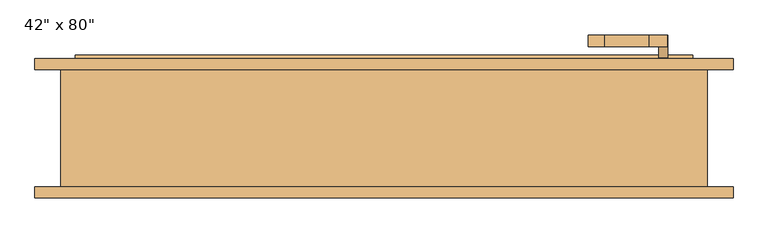
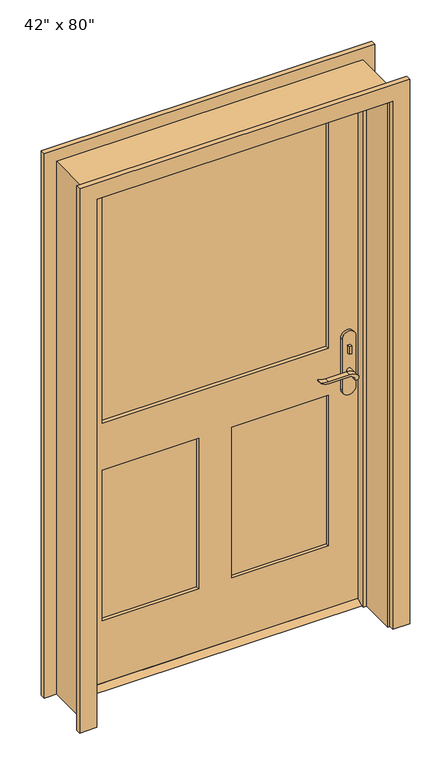
"""IFC4 building model written with IfcOpenShell, lengths in millimetres: door geometry."""

from ifc_helpers import new_model, si_unit, point, frame, frame_2d, origin, place, context, project, spatial, polyline, circle_curve, trimmed, segment, composite_curve, outline, extrude, faceted_brep, source, transform, mapped, element, save


def door_e0076512(model_context):
    return source(origin(), model_context, "Body", "SolidModel", [
        extrude(outline(polyline([(63.5, 12.7), (98.425, 12.7), (123.825, 0.0), (38.1, 0.0), (63.5, 12.7)])), frame((-533.4, 0.0, 0.0), z_axis=(1.0, 0.0, 0.0), x_axis=(0.0, 1.0, 0.0)), (0.0, 0.0, 1.0), 1066.8),
        extrude(outline(polyline([(487.6, 43.5), (477.6, 43.5), (477.6, 53.5), (487.6, 53.5), (487.6, 43.5)])), frame((0.0, 0.0, 981.9), z_axis=(0.0, 0.0, 1.0), x_axis=(1.0, 0.0, 0.0)), (0.0, 0.0, 1.0), 30.0),
        extrude(outline(composite_curve([segment(trimmed(circle_curve(frame_2d((996.9, 482.6)), 8.0), [point((996.9, 474.6))], [point((996.9, 490.6))], False, "CARTESIAN"), True, "CONTINUOUS"), segment(trimmed(circle_curve(frame_2d((996.9, 482.6)), 8.0), [point((996.9, 490.6))], [point((996.9, 474.6))], False, "CARTESIAN"), True, "CONTINUOUS")], self_intersect=False)), frame((0.0, 108.425, 0.0), z_axis=(0.0, 1.0, 0.0), x_axis=(0.0, 0.0, 1.0)), (0.0, 0.0, 1.0), 10.0),
        extrude(outline(composite_curve([segment(trimmed(circle_curve(frame_2d((897.1555521, 458.9324871)), 37.2832219), [point((919.0523287, 489.1081363))], [point((934.4, 457.2325667))], False, "CARTESIAN"), True, "CONTINUOUS"), segment(polyline([(934.4, 457.2325667), (934.4, 380.9564091)]), True, "CONTINUOUS"), segment(trimmed(circle_curve(frame_2d((1017.6850638, 381.0227909)), 83.2850902), [point((934.4, 380.9564091))], [point((939.4, 352.6))], True, "CARTESIAN"), True, "CONTINUOUS"), segment(polyline([(939.4, 352.6), (936.6135558, 352.6)]), True, "CONTINUOUS"), segment(trimmed(circle_curve(frame_2d((986.6709207, 384.5396612)), 59.3791355), [point((936.6135558, 352.6))], [point((927.4, 380.9564091))], False, "CARTESIAN"), True, "CONTINUOUS"), segment(polyline([(927.4, 380.9564091), (927.4, 457.2138099)]), True, "CONTINUOUS"), segment(trimmed(circle_curve(frame_2d((909.2738613, 457.2138099)), 18.1261387), [point((927.4, 457.2138099))], [point((914.4, 474.6))], True, "CARTESIAN"), True, "CONTINUOUS"), segment(trimmed(circle_curve(frame_2d((914.4, 482.6)), 8.0), [point((914.4, 474.6))], [point((919.0523287, 489.1081363))], False, "CARTESIAN"), True, "CONTINUOUS")], self_intersect=False)), frame((0.0, 3.5, 0.0), z_axis=(0.0, 1.0, 0.0), x_axis=(0.0, 0.0, 1.0)), (0.0, 0.0, 1.0), 20.0),
        extrude(outline(composite_curve([segment(trimmed(circle_curve(frame_2d((914.4, 482.6)), 8.0), [point((914.3999903, 474.6))], [point((919.0523287, 489.1081363))], False, "CARTESIAN"), True, "CONTINUOUS"), segment(trimmed(circle_curve(frame_2d((897.1555521, 458.9324871)), 37.2832219), [point((919.0523287, 489.1081363))], [point((934.4, 457.2325667))], False, "CARTESIAN"), True, "CONTINUOUS"), segment(polyline([(934.4, 457.2325667), (934.4, 380.9564091)]), True, "CONTINUOUS"), segment(trimmed(circle_curve(frame_2d((1017.6850638, 381.0227909)), 83.2850902), [point((934.4, 380.9564091))], [point((939.4, 352.6))], True, "CARTESIAN"), True, "CONTINUOUS"), segment(polyline([(939.4, 352.6), (936.6135558, 352.6)]), True, "CONTINUOUS"), segment(trimmed(circle_curve(frame_2d((986.6709207, 384.5396612)), 59.3791355), [point((936.6135558, 352.6))], [point((927.4, 380.9564091))], False, "CARTESIAN"), True, "CONTINUOUS"), segment(polyline([(927.4, 380.9564091), (927.4, 457.2138122)]), True, "CONTINUOUS"), segment(trimmed(circle_curve(frame_2d((909.2738682, 457.2138122)), 18.1261318), [point((927.4, 457.2138122))], [point((914.3999903, 474.6))], True, "CARTESIAN"), True, "CONTINUOUS")], self_intersect=False)), frame((0.0, 138.425, 0.0), z_axis=(0.0, 1.0, 0.0), x_axis=(0.0, 0.0, 1.0)), (0.0, 0.0, 1.0), 20.0),
        extrude(outline(composite_curve([segment(trimmed(circle_curve(frame_2d((914.4, 482.6)), 8.0), [point((914.4, 474.6))], [point((914.4, 490.6))], False, "CARTESIAN"), True, "CONTINUOUS"), segment(trimmed(circle_curve(frame_2d((914.4, 482.6)), 8.0), [point((914.4, 490.6))], [point((914.4, 474.6))], False, "CARTESIAN"), True, "CONTINUOUS")], self_intersect=False)), frame((0.0, 23.5, 0.0), z_axis=(0.0, 1.0, 0.0), x_axis=(0.0, 0.0, 1.0)), (0.0, 0.0, 1.0), 30.0),
        extrude(outline(composite_curve([segment(trimmed(circle_curve(frame_2d((914.4, 482.6)), 8.0), [point((914.4, 474.6))], [point((914.4, 490.6))], False, "CARTESIAN"), True, "CONTINUOUS"), segment(trimmed(circle_curve(frame_2d((914.4, 482.6)), 8.0), [point((914.4, 490.6))], [point((914.4, 474.6))], False, "CARTESIAN"), True, "CONTINUOUS")], self_intersect=False)), frame((0.0, 108.425, 0.0), z_axis=(0.0, 1.0, 0.0), x_axis=(0.0, 0.0, 1.0)), (0.0, 0.0, 1.0), 30.0),
        extrude(outline(composite_curve([segment(polyline([(844.4, 507.6), (1039.4, 507.6)]), True, "CONTINUOUS"), segment(trimmed(circle_curve(frame_2d((1039.4, 482.6)), 25.0), [point((1039.4, 507.6))], [point((1039.4, 457.6))], False, "CARTESIAN"), True, "CONTINUOUS"), segment(polyline([(1039.4, 457.6), (844.4, 457.6)]), True, "CONTINUOUS"), segment(trimmed(circle_curve(frame_2d((844.4, 482.6)), 25.0), [point((844.4, 457.6))], [point((844.4, 507.6))], False, "CARTESIAN"), True, "CONTINUOUS")], self_intersect=False)), frame((0.0, 53.5, 0.0), z_axis=(0.0, 1.0, 0.0), x_axis=(0.0, 0.0, 1.0)), (0.0, 0.0, 1.0), 10.0),
        extrude(outline(composite_curve([segment(polyline([(844.4, 507.6), (1039.4, 507.6)]), True, "CONTINUOUS"), segment(trimmed(circle_curve(frame_2d((1039.4, 482.6)), 25.0), [point((1039.4, 507.6))], [point((1039.4, 457.6))], False, "CARTESIAN"), True, "CONTINUOUS"), segment(polyline([(1039.4, 457.6), (844.4, 457.6)]), True, "CONTINUOUS"), segment(trimmed(circle_curve(frame_2d((844.4, 482.6)), 25.0), [point((844.4, 457.6))], [point((844.4, 507.6))], False, "CARTESIAN"), True, "CONTINUOUS")], self_intersect=False)), frame((0.0, 98.425, 0.0), z_axis=(0.0, 1.0, 0.0), x_axis=(0.0, 0.0, 1.0)), (0.0, 0.0, 1.0), 10.0),
        extrude(outline(polyline([(2032.0, -533.4), (12.7, -533.4), (12.7, 533.4), (2032.0, 533.4), (2032.0, -533.4)]), holes=[polyline([(1016.0, -412.75), (1911.35, -412.75), (1911.35, 412.75), (1016.0, 412.75), (1016.0, -412.75)]), polyline([(835.025, -60.325), (254.0, -60.325), (254.0, -412.75), (835.025, -412.75), (835.025, -60.325)]), polyline([(835.025, 412.75), (254.0, 412.75), (254.0, 60.325), (835.025, 60.325), (835.025, 412.75)])]), frame((0.0, 63.5, 0.0), z_axis=(0.0, 1.0, 0.0), x_axis=(0.0, 0.0, 1.0)), (0.0, 0.0, 1.0), 34.925),
        faceted_brep([(558.8, 98.425, 0.0), (558.8, -104.775, 0.0), (533.4, -104.775, 0.0), (533.4, 28.575, 0.0), (520.7, 28.575, 0.0), (520.7, 63.5, 0.0), (533.4, 63.5, 0.0), (533.4, 98.425, 0.0), (558.8, 98.425, 2057.4), (558.8, -104.775, 2057.4), (-558.8, -104.775, 2057.4), (-558.8, -104.775, 0.0), (-533.4, -104.775, 0.0), (-533.4, -104.775, 2032.0), (533.4, -104.775, 2032.0), (533.4, 28.575, 2032.0), (-533.4, 28.575, 2032.0), (-533.4, 28.575, 0.0), (-520.7, 28.575, 0.0), (-520.7, 28.575, 2019.3), (520.7, 28.575, 2019.3), (520.7, 63.5, 2019.3), (-520.7, 63.5, 2019.3), (-520.7, 63.5, 0.0), (-533.4, 63.5, 0.0), (-533.4, 63.5, 2032.0), (533.4, 63.5, 2032.0), (533.4, 98.425, 2032.0), (-533.4, 98.425, 2032.0), (-533.4, 98.425, 0.0), (-558.8, 98.425, 0.0), (-558.8, 98.425, 2057.4)], [[[0, 1, 2, 3, 4, 5, 6, 7]], [[1, 0, 8, 9]], [[2, 1, 9, 10, 11, 12, 13, 14]], [[3, 2, 14, 15]], [[4, 3, 15, 16, 17, 18, 19, 20]], [[5, 4, 20, 21]], [[6, 5, 21, 22, 23, 24, 25, 26]], [[7, 6, 26, 27]], [[0, 7, 27, 28, 29, 30, 31, 8]], [[9, 8, 31, 10]], [[15, 14, 13, 16]], [[21, 20, 19, 22]], [[27, 26, 25, 28]], [[30, 29, 24, 23, 18, 17, 12, 11]], [[10, 31, 30, 11]], [[16, 13, 12, 17]], [[22, 19, 18, 23]], [[28, 25, 24, 29]]]),
        extrude(outline(polyline([(-60.325, 75.1416667), (-412.75, 75.1416667), (-412.75, 86.7833333), (-60.325, 86.7833333), (-60.325, 75.1416667)])), frame((0.0, 0.0, 254.0), z_axis=(0.0, 0.0, 1.0), x_axis=(1.0, 0.0, 0.0)), (0.0, 0.0, 1.0), 581.025),
        extrude(outline(polyline([(412.75, 75.1416667), (60.325, 75.1416667), (60.325, 86.7833333), (412.75, 86.7833333), (412.75, 75.1416667)])), frame((0.0, 0.0, 254.0), z_axis=(0.0, 0.0, 1.0), x_axis=(1.0, 0.0, 0.0)), (0.0, 0.0, 1.0), 581.025),
        extrude(outline(polyline([(412.75, 77.47), (-412.75, 77.47), (-412.75, 84.455), (412.75, 84.455), (412.75, 77.47)])), frame((0.0, 0.0, 1016.0), z_axis=(0.0, 0.0, 1.0), x_axis=(1.0, 0.0, 0.0)), (0.0, 0.0, 1.0), 895.35),
        extrude(outline(polyline([(0.0, -603.25), (0.0, -539.75), (2038.35, -539.75), (2038.35, 539.75), (0.0, 539.75), (0.0, 603.25), (2101.85, 603.25), (2101.85, -603.25), (0.0, -603.25)])), frame((0.0, -123.825, 0.0), z_axis=(0.0, 1.0, 0.0), x_axis=(0.0, 0.0, 1.0)), (0.0, 0.0, 1.0), 19.05),
        extrude(outline(polyline([(0.0, -603.25), (0.0, -539.75), (2038.35, -539.75), (2038.35, 539.75), (0.0, 539.75), (0.0, 603.25), (2101.85, 603.25), (2101.85, -603.25), (0.0, -603.25)])), frame((0.0, 98.425, 0.0), z_axis=(0.0, 1.0, 0.0), x_axis=(0.0, 0.0, 1.0)), (0.0, 0.0, 1.0), 19.05),
    ])


if __name__ == "__main__":
    model = new_model("IFC4")
    model_context = context("Model", 3, world=origin())
    ifc_project = project(units=[si_unit("LENGTHUNIT", "METRE", prefix="MILLI")], contexts=[model_context])
    site = spatial("IfcSite", under=ifc_project)
    building = spatial("IfcBuilding", under=site)
    placement = place(None, origin())
    door_shape = door_e0076512(model_context)
    element("IfcDoor", 1, ObjectType="42\" x 80\"", at=placement, inside=building, context=model_context, shape_type="MappedRepresentation", body=[
        mapped(door_shape, transform((0.0, 0.0, 0.0), x_axis=(1.0, 0.0, 0.0), y_axis=(0.0, 1.0, 0.0), z_axis=(0.0, 0.0, 1.0))),
    ])
    save(model, "model.ifc")

# Revit data of these elements
# Type "42\" x 80\""
#   Type Mark = "8"
#   Assembly Code = "B2030100"
#   Analytic Construction = "French door, wood frame with single glass"
#   Top Rail = 0' - 4 3/4"
#   Threshold Offset [instance default] = 0' - 0 1/2"
#   Thickness = 0' - 1 3/8"
#   Thermal Resistance (R) = 1.0696 (h·ft²·°F)/BTU
#   Swing Angle [instance default] = 90.00°
#   Stiles = 0' - 4 3/4"
#   Rough Width = 3' - 8"
#   Rough Height = 6' - 9"
#   Lock Rail = 0' - 7 1/8"
#   Height = 6' - 8"
#   Width = 3' - 6"
#   Heat Transfer Coefficient (U) = 0.9350 BTU/(h·ft²·°F)
#   Door Offset [instance default] = 0' - 0"
#   Bottom Rail = 0' - 9 1/2"
#   Threshold [instance default] = yes
#   Function = 1
#   Exterior Trim [instance default] = yes
#   Trim Material = Cherry
#   Threshold Material = Cherry
#   Panel Material = Cherry
#   Glazing = Glass
#   Frame Material = Cherry
#   Door Handle Material = Aluminum
#   Visual Light Transmittance = 0
#   Solar Heat Gain Coefficient = 0
#   Wall Closure = (empty or 0)
#   Construction Type = (empty or 0)
# Element 1 (IfcDoor, "42\" x 80\"")
#   Materials on its faces: "Cherry", "Aluminum", "Glass"
# Materials
#   "Cherry": class "Wood", colour RGB 226 177 128, transparency 0, Description = "Prunus Serotina", Cost = 0
#   "Glass": class "Glass", colour RGB 0 128 192, transparency 0.75, Description = "Soda Lime Glass", Cost = 0
#   "Aluminum": class "Metal", colour RGB 247 247 247, transparency 0, Description = "Aluminum 6061", Cost = 0
